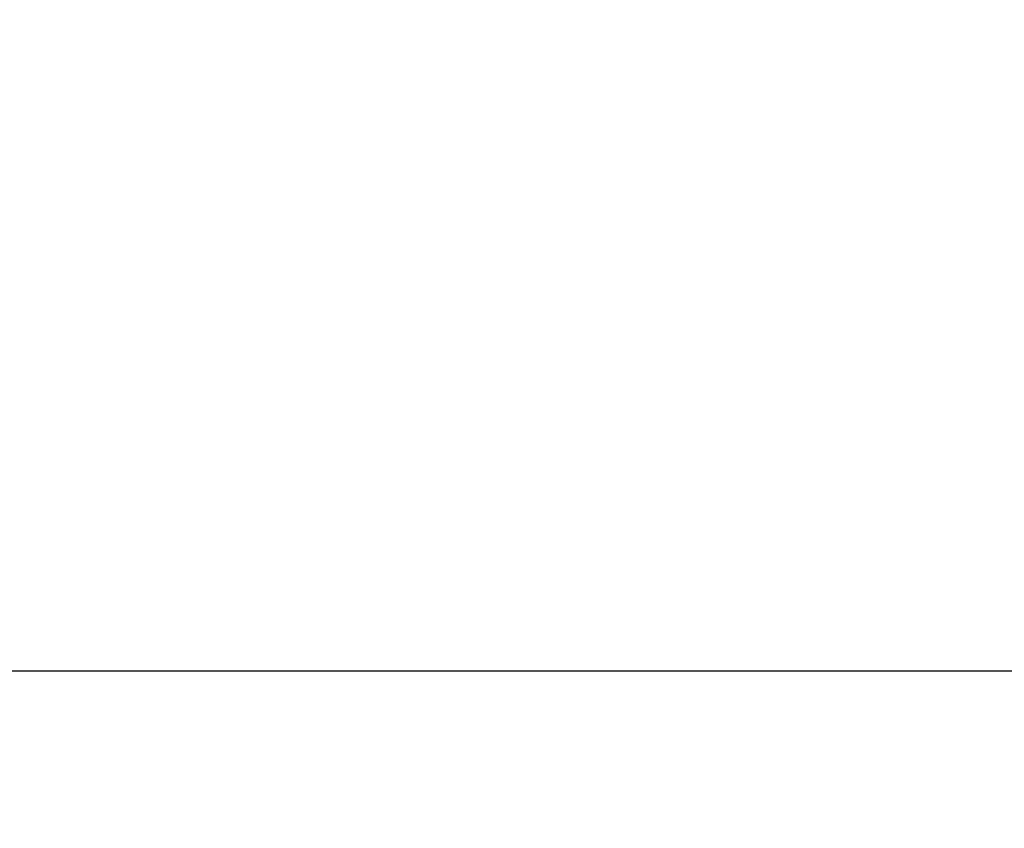
# Model space of a CAD drawing. Units: inches. Extents: x 1986 to 21484, y -1816 to 2016.
# Tile 38 of 85: x 2159.57 to 2174.94, y 1910.95 to 1923.57. Entities that reach past the tile are written whole.
import ezdxf

# ---------------------------------------------------------------- set-up
doc = ezdxf.new("R2010")
doc.units = ezdxf.units.IN
doc.layers.add('A-ANNO-DIMS', color=2, linetype='Continuous', lineweight=18)
doc.styles.get("Standard").update_dxf_attribs({"font": 'arial.ttf'})
doc.dimstyles.new('ISO-25', dxfattribs={"dimtxt": 8, "dimasz": 2.5, "dimexe": 1.25, "dimexo": 0.625, "dimtad": 1, "dimdec": 1, "dimlunit": 3, "dimtxsty": 'Standard', "dimcen": 2.5, "dimadec": 0, "dimazin": 0, "dimtfac": 1, "dimtdec": 1, "dimtmove": 0, "dimatfit": 3, "dimfxl": 1, "dimarcsym": 0})

# ---------------------------------------------------------------- blocks, each defined once
blk = doc.blocks.new('*D1')
at = {"layer": 'A-ANNO-DIMS', "color": 0, "lineweight": -2, "transparency": 16777216}
for p, q in [((2042.312, 1901.377), (2042.312, 1914.655)), ((2402.312, 1901.377), (2402.312, 1914.655)), ((2044.812, 1913.405), (2399.812, 1913.405))]:
    blk.add_line(p, q, dxfattribs=at)
at = {"layer": 'A-ANNO-DIMS', "color": 0, "transparency": 16777216}
for points in [[(2044.812, 1913.821), (2044.812, 1912.988), (2042.312, 1913.405)], [(2399.812, 1913.821), (2399.812, 1912.988), (2402.312, 1913.405)]]:
    blk.add_solid(points, dxfattribs=at)
at = {"layer": 'Defpoints', "color": 0, "transparency": 16777216}
for p in [(2402.312, 1913.405), (2042.312, 1900.752), (2402.312, 1900.752)]:
    blk.add_point(p, dxfattribs=at)
at = {"layer": 'A-ANNO-DIMS', "color": 0, "transparency": 16777216, "insert": (2222.312, 1918.117), "char_height": 8, "attachment_point": 5}
blk.add_mtext("30'", dxfattribs=at)

msp = doc.modelspace()

# ---------------------------------------------------------------- dimensions: what is measured, and where the dimension line sits
at = {"layer": 'A-ANNO-DIMS'}
dim = msp.add_linear_dim(base=(2402.312, 1913.405), p1=(2042.312, 1900.752), p2=(2402.312, 1900.752), dimstyle='ISO-25', override={"dimclrd": 0, "dimclre": 0, "dimclrt": 0}, dxfattribs=at)
dim.commit()
dim.dimension.update_dxf_attribs({"geometry": '*D1', "text_midpoint": (2222.312, 1918.117)})

doc.saveas('drawing.dxf')
